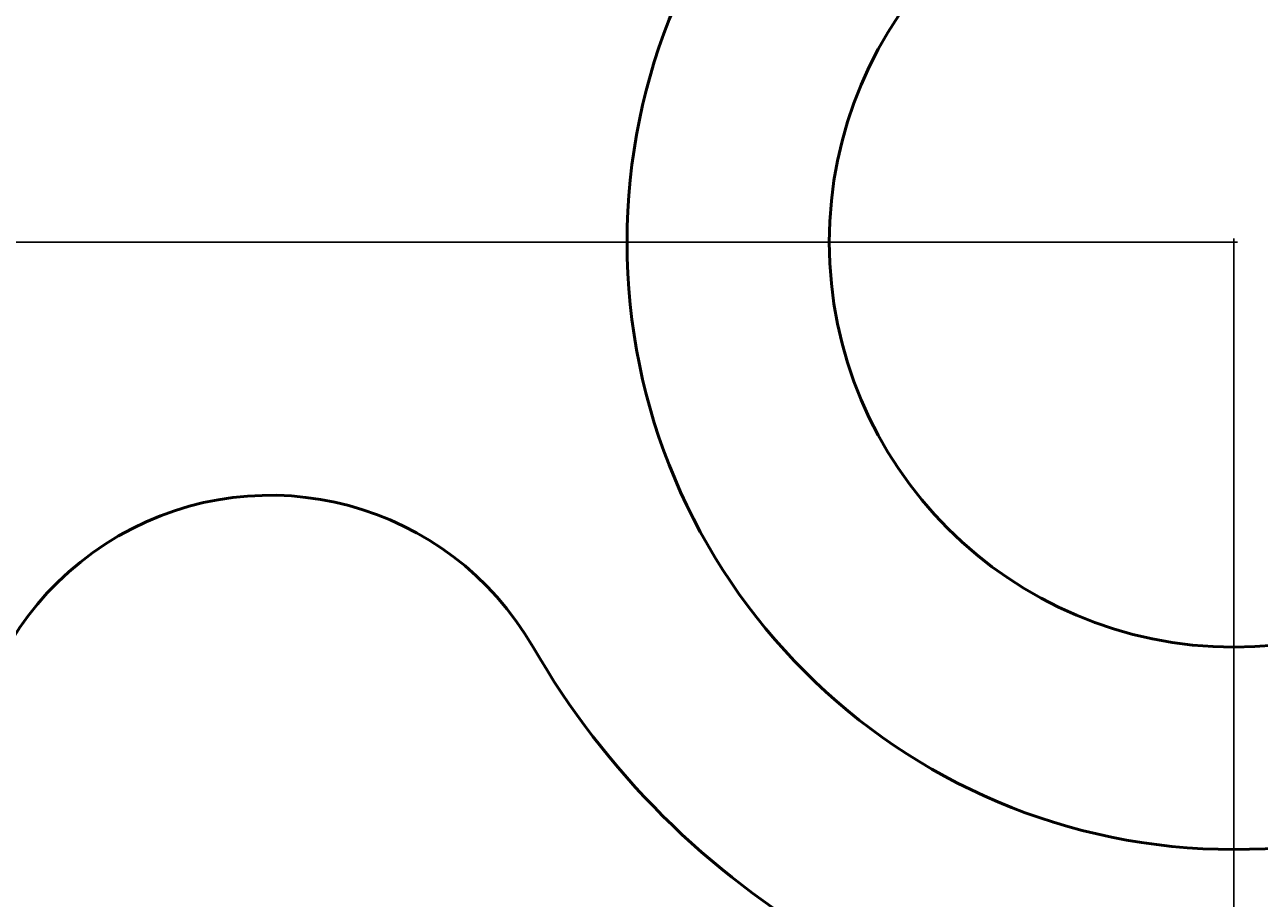
# Model space of a CAD drawing. Units: inches. Extents: x 413 to 622, y 326 to 447.
# Tile 3 of 15: x 443 to 473, y 370 to 392. Entities that reach past the tile are written whole.
import ezdxf

# ---------------------------------------------------------------- set-up
doc = ezdxf.new("R2010")
doc.units = ezdxf.units.IN
doc.header["$MEASUREMENT"] = 0
doc.layers.add('M-DIMS', color=2, linetype='Continuous', lineweight=18)
doc.layers.add('M-OUTL', color=7, linetype='Continuous', lineweight=50)
doc.styles.get("Standard").update_dxf_attribs({"font": 'arial.ttf'})
doc.dimstyles.get("Standard").update_dxf_attribs({"dimtxt": 0.18, "dimasz": 0.18, "dimexe": 0.18, "dimexo": 0.0625, "dimgap": 0.09, "dimtad": 0, "dimtih": 1, "dimtoh": 1, "dimdec": 4, "dimzin": 0, "dimdsep": 46, "dimtxsty": 'Standard', "dimcen": 0.09, "dimadec": 0, "dimazin": 0, "dimtfac": 1, "dimtdec": 4, "dimtofl": 0, "dimtmove": 0, "dimatfit": 3, "dimfxl": 1, "dimtolj": 1, "dimtzin": 0, "dimarcsym": 0})

# ---------------------------------------------------------------- blocks, each defined once
blk = doc.blocks.new('SPROCKET-HUB-BORE')
for radius in [15, 10]:
    blk.add_circle((15, 15), radius)
blk = doc.blocks.new('SPROCKET-WEB-SLOT')
for centre, radius, start, end in [((7.501, 21.25), 7.5, 30, 210), ((31.317, 35), 20, 210, 270)]:
    blk.add_arc(centre, radius, start, end)
blk = doc.blocks.new('*D10')
at = {"layer": 'Defpoints', "color": 0, "transparency": 16777216}
for p in [(413.283, 436.392), (472.684, 436.392), (472.684, 336.392)]:
    blk.add_point(p, dxfattribs=at)
at = {"layer": 'M-DIMS', "color": 0, "lineweight": -2, "transparency": 16777216}
for p, q in [((472.621, 436.392), (413.103, 436.392)), ((413.283, 436.212), (413.283, 386.573)), ((413.283, 336.572), (413.283, 386.21)), ((472.621, 336.392), (413.103, 336.392))]:
    blk.add_line(p, q, dxfattribs=at)
at = {"layer": 'M-DIMS', "color": 0, "transparency": 16777216}
for points in [[(413.253, 436.212), (413.313, 436.212), (413.283, 436.392)], [(413.253, 336.572), (413.313, 336.572), (413.283, 336.392)]]:
    blk.add_solid(points, dxfattribs=at)
at = {"layer": 'M-DIMS', "color": 0, "transparency": 16777216, "insert": (413.283, 386.392), "char_height": 0.18, "attachment_point": 5}
blk.add_mtext('\\A1;100', dxfattribs=at)
blk = doc.blocks.new('*D11')
at = {"layer": 'Defpoints', "color": 0, "transparency": 16777216}
for p in [(621.66, 446.422), (621.66, 388.074), (423.314, 378.888)]:
    blk.add_point(p, dxfattribs=at)
at = {"layer": 'M-DIMS', "color": 0, "lineweight": -2, "transparency": 16777216}
for p, q in [((423.314, 378.95), (423.314, 446.602)), ((621.66, 388.137), (621.66, 446.602)), ((423.494, 446.422), (522.031, 446.422)), ((621.48, 446.422), (522.943, 446.422))]:
    blk.add_line(p, q, dxfattribs=at)
at = {"layer": 'M-DIMS', "color": 0, "transparency": 16777216}
for points in [[(423.494, 446.452), (423.494, 446.392), (423.314, 446.422)], [(621.48, 446.452), (621.48, 446.392), (621.66, 446.422)]]:
    blk.add_solid(points, dxfattribs=at)
at = {"layer": 'M-DIMS', "color": 0, "transparency": 16777216, "insert": (522.487, 446.422), "char_height": 0.18, "attachment_point": 5}
blk.add_mtext('\\A1;198.35', dxfattribs=at)
blk = doc.blocks.new('*D12')
at = {"layer": 'Defpoints', "color": 0, "transparency": 16777216}
for p in [(472.684, 386.392), (592.684, 386.392), (592.684, 326.361)]:
    blk.add_point(p, dxfattribs=at)
at = {"layer": 'M-DIMS', "color": 0, "lineweight": -2, "transparency": 16777216}
for p, q in [((472.684, 386.329), (472.684, 326.181)), ((592.684, 386.329), (592.684, 326.181)), ((472.864, 326.361), (532.404, 326.361)), ((592.504, 326.361), (532.964, 326.361))]:
    blk.add_line(p, q, dxfattribs=at)
at = {"layer": 'M-DIMS', "color": 0, "transparency": 16777216}
for points in [[(472.864, 326.391), (472.864, 326.331), (472.684, 326.361)], [(592.504, 326.391), (592.504, 326.331), (592.684, 326.361)]]:
    blk.add_solid(points, dxfattribs=at)
at = {"layer": 'M-DIMS', "color": 0, "transparency": 16777216, "insert": (532.684, 326.361), "char_height": 0.18, "attachment_point": 5}
blk.add_mtext('\\A1;120', dxfattribs=at)
blk = doc.blocks.new('*D13')
at = {"layer": 'Defpoints', "color": 0, "transparency": 16777216}
for p in [(413.283, 431.392), (472.684, 431.392), (472.684, 386.392)]:
    blk.add_point(p, dxfattribs=at)
at = {"layer": 'M-DIMS', "color": 0, "lineweight": -2, "transparency": 16777216}
for p, q in [((472.621, 431.392), (413.103, 431.392)), ((413.283, 431.212), (413.283, 409.073)), ((413.283, 386.572), (413.283, 408.71)), ((472.621, 386.392), (413.103, 386.392))]:
    blk.add_line(p, q, dxfattribs=at)
at = {"layer": 'M-DIMS', "color": 0, "transparency": 16777216}
for points in [[(413.253, 431.212), (413.313, 431.212), (413.283, 431.392)], [(413.253, 386.572), (413.313, 386.572), (413.283, 386.392)]]:
    blk.add_solid(points, dxfattribs=at)
at = {"layer": 'M-DIMS', "color": 0, "transparency": 16777216, "insert": (413.283, 408.892), "char_height": 0.18, "attachment_point": 5}
blk.add_mtext('\\A1;45', dxfattribs=at)
blk = doc.blocks.new('*D24')
at = {"layer": 'Defpoints', "color": 0, "transparency": 16777216}
for p in [(432.684, 386.391), (512.684, 386.392)]:
    blk.add_point(p, dxfattribs=at)
at = {"layer": 'M-DIMS', "color": 0, "lineweight": -2, "transparency": 16777216}
for p, q in [((472.594, 386.392), (472.774, 386.392)), ((472.684, 386.302), (472.684, 386.482)), ((536.684, 386.392), (512.864, 386.392))]:
    blk.add_line(p, q, dxfattribs=at)
at = {"layer": 'M-DIMS', "color": 0, "transparency": 16777216}
blk.add_solid([(512.864, 386.422), (512.864, 386.362), (512.684, 386.392)], dxfattribs=at)
at = {"layer": 'M-DIMS', "color": 0, "transparency": 16777216, "insert": (537, 386.392), "char_height": 0.18, "attachment_point": 5}
blk.add_mtext('\\A1;∅80', dxfattribs=at)
blk = doc.blocks.new('*D26')
at = {"layer": 'Defpoints', "color": 0, "transparency": 16777216}
for p in [(459.693, 393.89), (485.675, 378.893)]:
    blk.add_point(p, dxfattribs=at)
at = {"layer": 'M-DIMS', "color": 0, "lineweight": -2, "transparency": 16777216}
for p, q in [((451.718, 398.39), (451.898, 398.39)), ((451.898, 398.39), (459.537, 393.98)), ((472.594, 386.392), (472.774, 386.392)), ((472.684, 386.302), (472.684, 386.482))]:
    blk.add_line(p, q, dxfattribs=at)
at = {"layer": 'M-DIMS', "color": 0, "transparency": 16777216}
blk.add_solid([(459.552, 394.006), (459.522, 393.954), (459.693, 393.89)], dxfattribs=at)
at = {"layer": 'M-DIMS', "color": 0, "transparency": 16777216, "insert": (451.211, 398.39), "char_height": 0.18, "attachment_point": 5}
blk.add_mtext('\\A1;2X ∅30', dxfattribs=at)
blk = doc.blocks.new('*D27')
at = {"layer": 'Defpoints', "color": 0, "transparency": 16777216}
for p in [(464.022, 391.39), (481.345, 381.393)]:
    blk.add_point(p, dxfattribs=at)
at = {"layer": 'M-DIMS', "color": 0, "lineweight": -2, "transparency": 16777216}
for p, q in [((472.594, 386.392), (472.774, 386.392)), ((472.684, 386.302), (472.684, 386.482)), ((486.542, 378.394), (481.501, 381.303)), ((486.722, 378.394), (486.542, 378.394))]:
    blk.add_line(p, q, dxfattribs=at)
at = {"layer": 'M-DIMS', "color": 0, "transparency": 16777216}
blk.add_solid([(481.516, 381.329), (481.486, 381.277), (481.345, 381.393)], dxfattribs=at)
at = {"layer": 'M-DIMS', "color": 0, "transparency": 16777216, "insert": (487.228, 378.394), "char_height": 0.18, "attachment_point": 5}
blk.add_mtext('\\A1;2X ∅20', dxfattribs=at)
blk = doc.blocks.new('*D28')
at = {"layer": 'Defpoints', "color": 0, "transparency": 16777216}
for p in [(455.184, 416.702), (472.684, 386.392)]:
    blk.add_point(p, dxfattribs=at)
at = {"layer": 'M-DIMS', "color": 0, "lineweight": -2, "transparency": 16777216}
for p, q in [((444.504, 434.889), (444.684, 434.889)), ((444.684, 434.889), (455.094, 416.858)), ((472.594, 386.392), (472.774, 386.392)), ((472.684, 386.302), (472.684, 386.482))]:
    blk.add_line(p, q, dxfattribs=at)
at = {"layer": 'M-DIMS', "color": 0, "transparency": 16777216}
blk.add_solid([(455.12, 416.873), (455.068, 416.843), (455.184, 416.702)], dxfattribs=at)
at = {"layer": 'M-DIMS', "color": 0, "transparency": 16777216, "insert": (444.005, 434.889), "char_height": 0.18, "attachment_point": 5}
blk.add_mtext('\\A1;3X R35', dxfattribs=at)
blk = doc.blocks.new('*D29')
at = {"layer": 'Defpoints', "color": 0, "transparency": 16777216}
for p in [(472.684, 386.392), (462.684, 369.071)]:
    blk.add_point(p, dxfattribs=at)
at = {"layer": 'M-DIMS', "color": 0, "lineweight": -2, "transparency": 16777216}
for p, q in [((472.594, 386.392), (472.774, 386.392)), ((472.684, 386.302), (472.684, 386.482)), ((456.684, 358.678), (462.594, 368.915)), ((456.504, 358.678), (456.684, 358.678))]:
    blk.add_line(p, q, dxfattribs=at)
at = {"layer": 'M-DIMS', "color": 0, "transparency": 16777216}
blk.add_solid([(462.568, 368.93), (462.62, 368.9), (462.684, 369.071)], dxfattribs=at)
at = {"layer": 'M-DIMS', "color": 0, "transparency": 16777216, "insert": (456.006, 358.678), "char_height": 0.18, "attachment_point": 5}
blk.add_mtext('\\A1;3X R20', dxfattribs=at)

msp = doc.modelspace()

# ---------------------------------------------------------------- linework, layer by layer
at = {"layer": 'M-OUTL'}
msp.add_circle((472.6836, 386.3915), 40, dxfattribs=at)

# ---------------------------------------------------------------- block references
for name, p in [('SPROCKET-HUB-BORE', (457.684, 371.392)), ('SPROCKET-WEB-SLOT', (441.367, 351.392))]:
    msp.add_blockref(name, p, dxfattribs=at)

# ---------------------------------------------------------------- dimensions: what is measured, and where the dimension line sits
at = {"layer": 'M-DIMS'}
for base, p1, p2, override, picture, middle in [((621.66, 446.422), (423.3136, 378.8878), (621.66, 388.0741), {"dimdec": 2, "dimlfac": 1, "dimrnd": 0, "dimzin": 0, "dimdsep": 46, "dimlunit": 2}, '*D11', (522.4868, 446.422)), ((592.6836, 326.361), (472.6836, 386.3915), (592.6836, 386.3915), {"dimdec": 0, "dimlfac": 1, "dimrnd": 0, "dimzin": 0, "dimdsep": 46, "dimlunit": 2}, '*D12', (532.6836, 326.361))]:
    dim = msp.add_linear_dim(base=base, p1=p1, p2=p2, dimstyle='Standard', override=override, dxfattribs=at)
    dim.commit()
    dim.dimension.update_dxf_attribs({"geometry": picture, "text_midpoint": middle})
for base, p1, p2, picture, middle in [((413.2831, 436.3915), (472.6836, 336.3915), (472.6836, 436.3915), '*D10', (413.2831, 386.3915)), ((413.2831, 431.3915), (472.6836, 386.3915), (472.6836, 431.3915), '*D13', (413.2831, 408.8915))]:
    dim = msp.add_linear_dim(base=base, p1=p1, p2=p2, angle=90, dimstyle='Standard', override={"dimdec": 0, "dimlfac": 1, "dimrnd": 0, "dimzin": 0, "dimdsep": 46, "dimlunit": 2}, dxfattribs=at)
    dim.commit()
    dim.dimension.update_dxf_attribs({"geometry": picture, "text_midpoint": middle})
for mpoint, picture, middle in [((455.1837, 416.7025), '*D28', (444.0048, 434.889)), ((462.6839, 369.0708), '*D29', (456.006, 358.6784))]:
    dim = msp.add_radius_dim(center=(472.6836, 386.3915), mpoint=mpoint, text='3X <>', dimstyle='Standard', override={"dimdec": 0, "dimlfac": 1, "dimrnd": 0, "dimzin": 0, "dimdsep": 46, "dimlunit": 2}, dxfattribs=at)
    dim.commit()
    dim.dimension.update_dxf_attribs({"geometry": picture, "text_midpoint": middle, "dimtype": 164})
for p1, p2, picture, middle in [((485.6746, 378.8925), (459.6926, 393.8905), '*D26', (451.2114, 398.3899)), ((464.0223, 391.3898), (481.3448, 381.3932), '*D27', (487.2283, 378.3943))]:
    dim = msp.add_diameter_dim_2p(p1=p1, p2=p2, text='2X <>', dimstyle='Standard', override={"dimdec": 0, "dimlfac": 1, "dimrnd": 0, "dimzin": 0, "dimdsep": 46, "dimlunit": 2}, dxfattribs=at)
    dim.commit()
    dim.dimension.update_dxf_attribs({"geometry": picture, "text_midpoint": middle, "dimtype": 163})
dim = msp.add_diameter_dim_2p(p1=(432.6836, 386.391), p2=(512.6836, 386.392), dimstyle='Standard', override={"dimdec": 0, "dimlfac": 1, "dimrnd": 0, "dimzin": 0, "dimdsep": 46, "dimlunit": 2}, dxfattribs=at)
dim.commit()
dim.dimension.update_dxf_attribs({"geometry": '*D24', "text_midpoint": (536.6836, 386.3923), "dimtype": 163})

doc.saveas('drawing.dxf')
